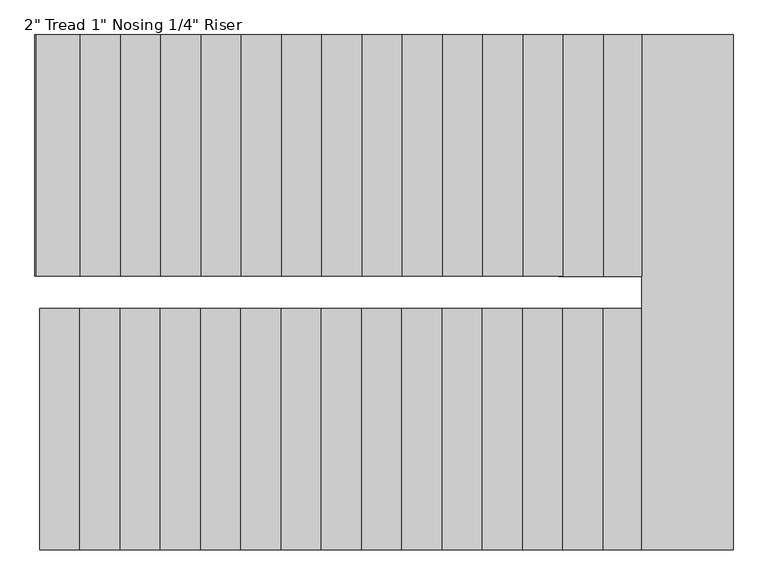
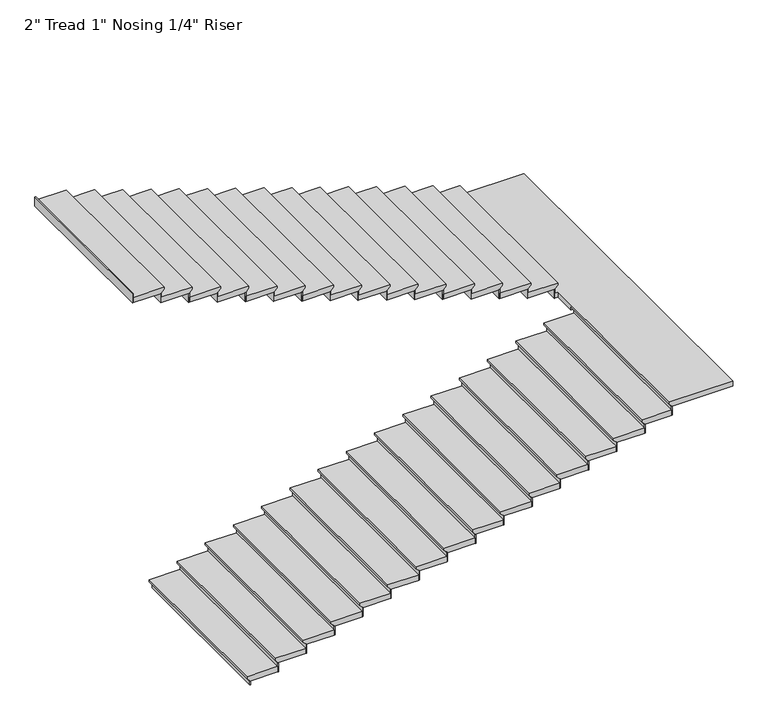
"""IFC4 building model written with IfcOpenShell, lengths in millimetres: stair flight geometry."""

from ifc_helpers import new_model, si_unit, origin, place, context, project, spatial, faceted_brep, source, transform, mapped, element, save


def stair_flight_242bbcd4(model_context):
    return source(origin(), model_context, "Body", "Brep", [
        faceted_brep([(1449.3932247, -2065.2659014, 6162.675), (1449.3932247, -2065.2659014, 6181.725), (1449.3932247, -541.2659014, 6181.725), (1449.3932247, -541.2659014, 6162.675), (1474.7932247, -2065.2659014, 6137.275), (1474.7932247, -541.2659014, 6137.275), (1726.3621616, -2065.2659014, 6181.725), (1726.3621616, -541.2659014, 6181.725), (1474.7932247, -541.2659014, 6130.925), (1726.3621616, -541.2659014, 6130.925), (1726.3621616, -2065.2659014, 6130.925), (1474.7932247, -2065.2659014, 6130.925)], [[[0, 1, 2, 3]], [[4, 0, 3, 5]], [[2, 1, 6, 7]], [[8, 9, 10, 11]], [[2, 7, 9, 8, 5, 3]], [[8, 11, 4, 5]], [[6, 1, 0, 4, 11, 10]], [[7, 6, 10, 9]]]),
        faceted_brep([(1474.7932247, -2065.2659014, 6130.925), (1474.7932247, -2065.2659014, 6096.0), (1481.1432247, -2065.2659014, 6096.0), (1481.1432247, -2065.2659014, 6130.925), (1474.7932247, -541.2659014, 6130.925), (1481.1432247, -541.2659014, 6130.925), (1481.1432247, -541.2659014, 6096.0), (1474.7932247, -541.2659014, 6096.0)], [[[0, 1, 2, 3]], [[4, 5, 6, 7]], [[1, 0, 4, 7]], [[2, 1, 7, 6]], [[3, 2, 6, 5]], [[0, 3, 5, 4]]]),
        faceted_brep([(1726.3621616, -2065.2659014, 6216.65), (1726.3621616, -2065.2659014, 6130.925), (1732.7121616, -2065.2659014, 6130.925), (1732.7121616, -2065.2659014, 6216.65), (1726.3621616, -541.2659014, 6216.65), (1732.7121616, -541.2659014, 6216.65), (1732.7121616, -541.2659014, 6130.925), (1726.3621616, -541.2659014, 6130.925)], [[[0, 1, 2, 3]], [[4, 5, 6, 7]], [[1, 0, 4, 7]], [[2, 1, 7, 6]], [[3, 2, 6, 5]], [[0, 3, 5, 4]]]),
        faceted_brep([(1700.9621616, -541.2659014, 6267.45), (1700.9621616, -2065.2659014, 6267.45), (1980.3621616, -2065.2659014, 6267.45), (1980.3621616, -541.2659014, 6267.45), (1726.3621616, -541.2659014, 6216.65), (1980.3621616, -541.2659014, 6216.65), (1980.3621616, -2065.2659014, 6216.65), (1726.3621616, -2065.2659014, 6216.65), (1726.3621616, -541.2659014, 6223.0), (1700.9621616, -541.2659014, 6248.4), (1726.3621616, -2065.2659014, 6223.0), (1700.9621616, -2065.2659014, 6248.4)], [[[0, 1, 2, 3]], [[4, 5, 6, 7]], [[0, 3, 5, 4, 8, 9]], [[4, 7, 10, 8]], [[2, 1, 11, 10, 7, 6]], [[3, 2, 6, 5]], [[11, 1, 0, 9]], [[10, 11, 9, 8]]]),
        faceted_brep([(1980.3621616, -2065.2659014, 6302.375), (1980.3621616, -2065.2659014, 6216.65), (1986.7121616, -2065.2659014, 6216.65), (1986.7121616, -2065.2659014, 6302.375), (1980.3621616, -541.2659014, 6302.375), (1986.7121616, -541.2659014, 6302.375), (1986.7121616, -541.2659014, 6216.65), (1980.3621616, -541.2659014, 6216.65)], [[[0, 1, 2, 3]], [[4, 5, 6, 7]], [[1, 0, 4, 7]], [[2, 1, 7, 6]], [[3, 2, 6, 5]], [[0, 3, 5, 4]]]),
        faceted_brep([(1954.9621616, -541.2659014, 6353.175), (1954.9621616, -2065.2659014, 6353.175), (2234.3621616, -2065.2659014, 6353.175), (2234.3621616, -541.2659014, 6353.175), (1980.3621616, -541.2659014, 6302.375), (2234.3621616, -541.2659014, 6302.375), (2234.3621616, -2065.2659014, 6302.375), (1980.3621616, -2065.2659014, 6302.375), (1980.3621616, -541.2659014, 6308.725), (1954.9621616, -541.2659014, 6334.125), (1980.3621616, -2065.2659014, 6308.725), (1954.9621616, -2065.2659014, 6334.125)], [[[0, 1, 2, 3]], [[4, 5, 6, 7]], [[0, 3, 5, 4, 8, 9]], [[4, 7, 10, 8]], [[2, 1, 11, 10, 7, 6]], [[3, 2, 6, 5]], [[11, 1, 0, 9]], [[10, 11, 9, 8]]]),
        faceted_brep([(2234.3621616, -2065.2659014, 6388.1), (2234.3621616, -2065.2659014, 6302.375), (2240.7121616, -2065.2659014, 6302.375), (2240.7121616, -2065.2659014, 6388.1), (2234.3621616, -541.2659014, 6388.1), (2240.7121616, -541.2659014, 6388.1), (2240.7121616, -541.2659014, 6302.375), (2234.3621616, -541.2659014, 6302.375)], [[[0, 1, 2, 3]], [[4, 5, 6, 7]], [[1, 0, 4, 7]], [[2, 1, 7, 6]], [[3, 2, 6, 5]], [[0, 3, 5, 4]]]),
        faceted_brep([(2208.9621616, -541.2659014, 6438.9), (2208.9621616, -2065.2659014, 6438.9), (2488.3621616, -2065.2659014, 6438.9), (2488.3621616, -541.2659014, 6438.9), (2234.3621616, -541.2659014, 6388.1), (2488.3621616, -541.2659014, 6388.1), (2488.3621616, -2065.2659014, 6388.1), (2234.3621616, -2065.2659014, 6388.1), (2234.3621616, -541.2659014, 6394.45), (2208.9621616, -541.2659014, 6419.85), (2234.3621616, -2065.2659014, 6394.45), (2208.9621616, -2065.2659014, 6419.85)], [[[0, 1, 2, 3]], [[4, 5, 6, 7]], [[0, 3, 5, 4, 8, 9]], [[4, 7, 10, 8]], [[2, 1, 11, 10, 7, 6]], [[3, 2, 6, 5]], [[11, 1, 0, 9]], [[10, 11, 9, 8]]]),
        faceted_brep([(2488.3621616, -2065.2659014, 6473.825), (2488.3621616, -2065.2659014, 6388.1), (2494.7121616, -2065.2659014, 6388.1), (2494.7121616, -2065.2659014, 6473.825), (2488.3621616, -541.2659014, 6473.825), (2494.7121616, -541.2659014, 6473.825), (2494.7121616, -541.2659014, 6388.1), (2488.3621616, -541.2659014, 6388.1)], [[[0, 1, 2, 3]], [[4, 5, 6, 7]], [[1, 0, 4, 7]], [[2, 1, 7, 6]], [[3, 2, 6, 5]], [[0, 3, 5, 4]]]),
        faceted_brep([(2462.9621616, -541.2659014, 6524.625), (2462.9621616, -2065.2659014, 6524.625), (2742.3621616, -2065.2659014, 6524.625), (2742.3621616, -541.2659014, 6524.625), (2488.3621616, -541.2659014, 6473.825), (2742.3621616, -541.2659014, 6473.825), (2742.3621616, -2065.2659014, 6473.825), (2488.3621616, -2065.2659014, 6473.825), (2488.3621616, -541.2659014, 6480.175), (2462.9621616, -541.2659014, 6505.575), (2488.3621616, -2065.2659014, 6480.175), (2462.9621616, -2065.2659014, 6505.575)], [[[0, 1, 2, 3]], [[4, 5, 6, 7]], [[0, 3, 5, 4, 8, 9]], [[4, 7, 10, 8]], [[2, 1, 11, 10, 7, 6]], [[3, 2, 6, 5]], [[11, 1, 0, 9]], [[10, 11, 9, 8]]]),
        faceted_brep([(2742.3621616, -2065.2659014, 6559.55), (2742.3621616, -2065.2659014, 6473.825), (2748.7121616, -2065.2659014, 6473.825), (2748.7121616, -2065.2659014, 6559.55), (2742.3621616, -541.2659014, 6559.55), (2748.7121616, -541.2659014, 6559.55), (2748.7121616, -541.2659014, 6473.825), (2742.3621616, -541.2659014, 6473.825)], [[[0, 1, 2, 3]], [[4, 5, 6, 7]], [[1, 0, 4, 7]], [[2, 1, 7, 6]], [[3, 2, 6, 5]], [[0, 3, 5, 4]]]),
        faceted_brep([(2716.9621616, -541.2659014, 6610.35), (2716.9621616, -2065.2659014, 6610.35), (2996.3621616, -2065.2659014, 6610.35), (2996.3621616, -541.2659014, 6610.35), (2742.3621616, -541.2659014, 6559.55), (2996.3621616, -541.2659014, 6559.55), (2996.3621616, -2065.2659014, 6559.55), (2742.3621616, -2065.2659014, 6559.55), (2742.3621616, -541.2659014, 6565.9), (2716.9621616, -541.2659014, 6591.3), (2742.3621616, -2065.2659014, 6565.9), (2716.9621616, -2065.2659014, 6591.3)], [[[0, 1, 2, 3]], [[4, 5, 6, 7]], [[0, 3, 5, 4, 8, 9]], [[4, 7, 10, 8]], [[2, 1, 11, 10, 7, 6]], [[3, 2, 6, 5]], [[11, 1, 0, 9]], [[10, 11, 9, 8]]]),
        faceted_brep([(2996.3621616, -2065.2659014, 6645.275), (2996.3621616, -2065.2659014, 6559.55), (3002.7121616, -2065.2659014, 6559.55), (3002.7121616, -2065.2659014, 6645.275), (2996.3621616, -541.2659014, 6645.275), (3002.7121616, -541.2659014, 6645.275), (3002.7121616, -541.2659014, 6559.55), (2996.3621616, -541.2659014, 6559.55)], [[[0, 1, 2, 3]], [[4, 5, 6, 7]], [[1, 0, 4, 7]], [[2, 1, 7, 6]], [[3, 2, 6, 5]], [[0, 3, 5, 4]]]),
        faceted_brep([(2970.9621616, -541.2659014, 6696.075), (2970.9621616, -2065.2659014, 6696.075), (3250.3621616, -2065.2659014, 6696.075), (3250.3621616, -541.2659014, 6696.075), (2996.3621616, -541.2659014, 6645.275), (3250.3621616, -541.2659014, 6645.275), (3250.3621616, -2065.2659014, 6645.275), (2996.3621616, -2065.2659014, 6645.275), (2996.3621616, -541.2659014, 6651.625), (2970.9621616, -541.2659014, 6677.025), (2996.3621616, -2065.2659014, 6651.625), (2970.9621616, -2065.2659014, 6677.025)], [[[0, 1, 2, 3]], [[4, 5, 6, 7]], [[0, 3, 5, 4, 8, 9]], [[4, 7, 10, 8]], [[2, 1, 11, 10, 7, 6]], [[3, 2, 6, 5]], [[11, 1, 0, 9]], [[10, 11, 9, 8]]]),
        faceted_brep([(3250.3621616, -2065.2659014, 6731.0), (3250.3621616, -2065.2659014, 6645.275), (3256.7121616, -2065.2659014, 6645.275), (3256.7121616, -2065.2659014, 6731.0), (3250.3621616, -541.2659014, 6731.0), (3256.7121616, -541.2659014, 6731.0), (3256.7121616, -541.2659014, 6645.275), (3250.3621616, -541.2659014, 6645.275)], [[[0, 1, 2, 3]], [[4, 5, 6, 7]], [[1, 0, 4, 7]], [[2, 1, 7, 6]], [[3, 2, 6, 5]], [[0, 3, 5, 4]]]),
        faceted_brep([(3224.9621616, -541.2659014, 6781.8), (3224.9621616, -2065.2659014, 6781.8), (3504.3621616, -2065.2659014, 6781.8), (3504.3621616, -541.2659014, 6781.8), (3250.3621616, -541.2659014, 6731.0), (3504.3621616, -541.2659014, 6731.0), (3504.3621616, -2065.2659014, 6731.0), (3250.3621616, -2065.2659014, 6731.0), (3250.3621616, -541.2659014, 6737.35), (3224.9621616, -541.2659014, 6762.75), (3250.3621616, -2065.2659014, 6737.35), (3224.9621616, -2065.2659014, 6762.75)], [[[0, 1, 2, 3]], [[4, 5, 6, 7]], [[0, 3, 5, 4, 8, 9]], [[4, 7, 10, 8]], [[2, 1, 11, 10, 7, 6]], [[3, 2, 6, 5]], [[11, 1, 0, 9]], [[10, 11, 9, 8]]]),
        faceted_brep([(3504.3621616, -2065.2659014, 6816.725), (3504.3621616, -2065.2659014, 6731.0), (3510.7121616, -2065.2659014, 6731.0), (3510.7121616, -2065.2659014, 6816.725), (3504.3621616, -541.2659014, 6816.725), (3510.7121616, -541.2659014, 6816.725), (3510.7121616, -541.2659014, 6731.0), (3504.3621616, -541.2659014, 6731.0)], [[[0, 1, 2, 3]], [[4, 5, 6, 7]], [[1, 0, 4, 7]], [[2, 1, 7, 6]], [[3, 2, 6, 5]], [[0, 3, 5, 4]]]),
        faceted_brep([(3478.9621616, -541.2659014, 6867.525), (3478.9621616, -2065.2659014, 6867.525), (3758.3621616, -2065.2659014, 6867.525), (3758.3621616, -541.2659014, 6867.525), (3504.3621616, -541.2659014, 6816.725), (3758.3621616, -541.2659014, 6816.725), (3758.3621616, -2065.2659014, 6816.725), (3504.3621616, -2065.2659014, 6816.725), (3504.3621616, -541.2659014, 6823.075), (3478.9621616, -541.2659014, 6848.475), (3504.3621616, -2065.2659014, 6823.075), (3478.9621616, -2065.2659014, 6848.475)], [[[0, 1, 2, 3]], [[4, 5, 6, 7]], [[0, 3, 5, 4, 8, 9]], [[4, 7, 10, 8]], [[2, 1, 11, 10, 7, 6]], [[3, 2, 6, 5]], [[11, 1, 0, 9]], [[10, 11, 9, 8]]]),
        faceted_brep([(3758.3621616, -2065.2659014, 6902.45), (3758.3621616, -2065.2659014, 6816.725), (3764.7121616, -2065.2659014, 6816.725), (3764.7121616, -2065.2659014, 6902.45), (3758.3621616, -541.2659014, 6902.45), (3764.7121616, -541.2659014, 6902.45), (3764.7121616, -541.2659014, 6816.725), (3758.3621616, -541.2659014, 6816.725)], [[[0, 1, 2, 3]], [[4, 5, 6, 7]], [[1, 0, 4, 7]], [[2, 1, 7, 6]], [[3, 2, 6, 5]], [[0, 3, 5, 4]]]),
        faceted_brep([(3732.9621616, -541.2659014, 6953.25), (3732.9621616, -2065.2659014, 6953.25), (4012.3621616, -2065.2659014, 6953.25), (4012.3621616, -541.2659014, 6953.25), (3758.3621616, -541.2659014, 6902.45), (4012.3621616, -541.2659014, 6902.45), (4012.3621616, -2065.2659014, 6902.45), (3758.3621616, -2065.2659014, 6902.45), (3758.3621616, -541.2659014, 6908.8), (3732.9621616, -541.2659014, 6934.2), (3758.3621616, -2065.2659014, 6908.8), (3732.9621616, -2065.2659014, 6934.2)], [[[0, 1, 2, 3]], [[4, 5, 6, 7]], [[0, 3, 5, 4, 8, 9]], [[4, 7, 10, 8]], [[2, 1, 11, 10, 7, 6]], [[3, 2, 6, 5]], [[11, 1, 0, 9]], [[10, 11, 9, 8]]]),
        faceted_brep([(4012.3621616, -2065.2659014, 6988.175), (4012.3621616, -2065.2659014, 6902.45), (4018.7121616, -2065.2659014, 6902.45), (4018.7121616, -2065.2659014, 6988.175), (4012.3621616, -541.2659014, 6988.175), (4018.7121616, -541.2659014, 6988.175), (4018.7121616, -541.2659014, 6902.45), (4012.3621616, -541.2659014, 6902.45)], [[[0, 1, 2, 3]], [[4, 5, 6, 7]], [[1, 0, 4, 7]], [[2, 1, 7, 6]], [[3, 2, 6, 5]], [[0, 3, 5, 4]]]),
        faceted_brep([(3986.9621616, -541.2659014, 7038.975), (3986.9621616, -2065.2659014, 7038.975), (4266.3621616, -2065.2659014, 7038.975), (4266.3621616, -541.2659014, 7038.975), (4012.3621616, -541.2659014, 6988.175), (4266.3621616, -541.2659014, 6988.175), (4266.3621616, -2065.2659014, 6988.175), (4012.3621616, -2065.2659014, 6988.175), (4012.3621616, -541.2659014, 6994.525), (3986.9621616, -541.2659014, 7019.925), (4012.3621616, -2065.2659014, 6994.525), (3986.9621616, -2065.2659014, 7019.925)], [[[0, 1, 2, 3]], [[4, 5, 6, 7]], [[0, 3, 5, 4, 8, 9]], [[4, 7, 10, 8]], [[2, 1, 11, 10, 7, 6]], [[3, 2, 6, 5]], [[11, 1, 0, 9]], [[10, 11, 9, 8]]]),
        faceted_brep([(4266.3621616, -2065.2659014, 7073.9), (4266.3621616, -2065.2659014, 6988.175), (4272.7121616, -2065.2659014, 6988.175), (4272.7121616, -2065.2659014, 7073.9), (4266.3621616, -541.2659014, 7073.9), (4272.7121616, -541.2659014, 7073.9), (4272.7121616, -541.2659014, 6988.175), (4266.3621616, -541.2659014, 6988.175)], [[[0, 1, 2, 3]], [[4, 5, 6, 7]], [[1, 0, 4, 7]], [[2, 1, 7, 6]], [[3, 2, 6, 5]], [[0, 3, 5, 4]]]),
        faceted_brep([(4240.9621616, -541.2659014, 7124.7), (4240.9621616, -2065.2659014, 7124.7), (4520.3621616, -2065.2659014, 7124.7), (4520.3621616, -541.2659014, 7124.7), (4266.3621616, -541.2659014, 7073.9), (4520.3621616, -541.2659014, 7073.9), (4520.3621616, -2065.2659014, 7073.9), (4266.3621616, -2065.2659014, 7073.9), (4266.3621616, -541.2659014, 7080.25), (4240.9621616, -541.2659014, 7105.65), (4266.3621616, -2065.2659014, 7080.25), (4240.9621616, -2065.2659014, 7105.65)], [[[0, 1, 2, 3]], [[4, 5, 6, 7]], [[0, 3, 5, 4, 8, 9]], [[4, 7, 10, 8]], [[2, 1, 11, 10, 7, 6]], [[3, 2, 6, 5]], [[11, 1, 0, 9]], [[10, 11, 9, 8]]]),
        faceted_brep([(4520.3621616, -2065.2659014, 7159.625), (4520.3621616, -2065.2659014, 7073.9), (4526.7121616, -2065.2659014, 7073.9), (4526.7121616, -2065.2659014, 7159.625), (4520.3621616, -541.2659014, 7159.625), (4526.7121616, -541.2659014, 7159.625), (4526.7121616, -541.2659014, 7073.9), (4520.3621616, -541.2659014, 7073.9)], [[[0, 1, 2, 3]], [[4, 5, 6, 7]], [[1, 0, 4, 7]], [[2, 1, 7, 6]], [[3, 2, 6, 5]], [[0, 3, 5, 4]]]),
        faceted_brep([(4494.9621616, -541.2659014, 7210.425), (4494.9621616, -2065.2659014, 7210.425), (4774.3621616, -2065.2659014, 7210.425), (4774.3621616, -541.2659014, 7210.425), (4520.3621616, -541.2659014, 7159.625), (4774.3621616, -541.2659014, 7159.625), (4774.3621616, -2065.2659014, 7159.625), (4520.3621616, -2065.2659014, 7159.625), (4520.3621616, -541.2659014, 7165.975), (4494.9621616, -541.2659014, 7191.375), (4520.3621616, -2065.2659014, 7165.975), (4494.9621616, -2065.2659014, 7191.375)], [[[0, 1, 2, 3]], [[4, 5, 6, 7]], [[0, 3, 5, 4, 8, 9]], [[4, 7, 10, 8]], [[2, 1, 11, 10, 7, 6]], [[3, 2, 6, 5]], [[11, 1, 0, 9]], [[10, 11, 9, 8]]]),
        faceted_brep([(4774.3621616, -2065.2659014, 7245.35), (4774.3621616, -2065.2659014, 7159.625), (4780.7121616, -2065.2659014, 7159.625), (4780.7121616, -2065.2659014, 7245.35), (4774.3621616, -541.2659014, 7245.35), (4780.7121616, -541.2659014, 7245.35), (4780.7121616, -541.2659014, 7159.625), (4774.3621616, -541.2659014, 7159.625)], [[[0, 1, 2, 3]], [[4, 5, 6, 7]], [[1, 0, 4, 7]], [[2, 1, 7, 6]], [[3, 2, 6, 5]], [[0, 3, 5, 4]]]),
        faceted_brep([(4748.9621616, -541.2659014, 7296.15), (4748.9621616, -2065.2659014, 7296.15), (5028.3621616, -2065.2659014, 7296.15), (5028.3621616, -541.2659014, 7296.15), (4774.3621616, -541.2659014, 7245.35), (5028.3621616, -541.2659014, 7245.35), (5028.3621616, -2065.2659014, 7245.35), (4774.3621616, -2065.2659014, 7245.35), (4774.3621616, -541.2659014, 7251.7), (4748.9621616, -541.2659014, 7277.1), (4774.3621616, -2065.2659014, 7251.7), (4748.9621616, -2065.2659014, 7277.1)], [[[0, 1, 2, 3]], [[4, 5, 6, 7]], [[0, 3, 5, 4, 8, 9]], [[4, 7, 10, 8]], [[2, 1, 11, 10, 7, 6]], [[3, 2, 6, 5]], [[11, 1, 0, 9]], [[10, 11, 9, 8]]]),
        faceted_brep([(5028.3621616, -2065.2659014, 7331.075), (5028.3621616, -2065.2659014, 7245.35), (5034.7121616, -2065.2659014, 7245.35), (5034.7121616, -2065.2659014, 7331.075), (5028.3621616, -541.2659014, 7331.075), (5034.7121616, -541.2659014, 7331.075), (5034.7121616, -541.2659014, 7245.35), (5028.3621616, -541.2659014, 7245.35)], [[[0, 1, 2, 3]], [[4, 5, 6, 7]], [[1, 0, 4, 7]], [[2, 1, 7, 6]], [[3, 2, 6, 5]], [[0, 3, 5, 4]]]),
        faceted_brep([(5002.9621616, -541.2659014, 7381.875), (5002.9621616, -2065.2659014, 7381.875), (5272.0669505, -2065.2659014, 7381.875), (5272.0669505, -541.2659014, 7381.875), (5028.3621616, -541.2659014, 7331.075), (5272.0669505, -541.2659014, 7331.075), (5272.0669505, -2065.2659014, 7331.075), (5028.3621616, -2065.2659014, 7331.075), (5028.3621616, -541.2659014, 7337.425), (5002.9621616, -541.2659014, 7362.825), (5028.3621616, -2065.2659014, 7337.425), (5002.9621616, -2065.2659014, 7362.825)], [[[0, 1, 2, 3]], [[4, 5, 6, 7]], [[0, 3, 5, 4, 8, 9]], [[4, 7, 10, 8]], [[2, 1, 11, 10, 7, 6]], [[3, 2, 6, 5]], [[11, 1, 0, 9]], [[10, 11, 9, 8]]]),
        faceted_brep([(5272.0669505, -2065.2659014, 7416.8), (5272.0669505, -2065.2659014, 7331.075), (5278.4169505, -2065.2659014, 7331.075), (5278.4169505, -2065.2659014, 7416.8), (5272.0669505, -541.2659014, 7416.8), (5278.4169505, -541.2659014, 7416.8), (5278.4169505, -541.2659014, 7331.075), (5272.0669505, -541.2659014, 7331.075)], [[[0, 1, 2, 3]], [[4, 5, 6, 7]], [[1, 0, 4, 7]], [[2, 1, 7, 6]], [[3, 2, 6, 5]], [[0, 3, 5, 4]]]),
        faceted_brep([(5221.2669505, -337.9910016, 7467.6), (5246.6669505, -337.9910016, 7467.6), (5246.6669505, -2065.2659014, 7467.6), (5822.2548051, -2065.2659014, 7467.6), (5822.2548051, 1185.9340986, 7467.6), (5221.2669505, 1185.9340986, 7467.6), (5246.6669505, -337.9910016, 7416.8), (5221.2669505, -337.9910016, 7416.8), (5221.2669505, 1185.9340986, 7416.8), (5822.2548051, 1185.9340986, 7416.8), (5822.2548051, -2065.2659014, 7416.8), (5272.0669505, -2065.2659014, 7416.8), (5272.0669505, -541.2659014, 7416.8), (5246.6669505, -541.2659014, 7416.8), (5246.6669505, -541.2659014, 7448.55), (5246.6669505, -2065.2659014, 7448.55), (5272.0669505, -541.2659014, 7423.15), (5272.0669505, -2065.2659014, 7423.15)], [[[0, 1, 2, 3, 4, 5]], [[6, 7, 8, 9, 10, 11, 12, 13]], [[1, 0, 7, 6]], [[2, 1, 6, 13, 14, 15]], [[13, 12, 16, 14]], [[12, 11, 17, 16]], [[3, 2, 15, 17, 11, 10]], [[4, 3, 10, 9]], [[5, 4, 9, 8]], [[0, 5, 8, 7]], [[17, 15, 14, 16]]]),
        faceted_brep([(5221.2669505, 1185.9340986, 7502.525), (5221.2669505, 1185.9340986, 7416.8), (5214.9169505, 1185.9340986, 7416.8), (5214.9169505, 1185.9340986, 7502.525), (5221.2669505, -337.9910016, 7502.525), (5214.9169505, -337.9910016, 7502.525), (5214.9169505, -337.9910016, 7416.8), (5221.2669505, -337.9910016, 7416.8)], [[[0, 1, 2, 3]], [[4, 5, 6, 7]], [[1, 0, 4, 7]], [[2, 1, 7, 6]], [[3, 2, 6, 5]], [[0, 3, 5, 4]]]),
        faceted_brep([(5246.6669505, -337.9910016, 7553.325), (5246.6669505, 1185.9340986, 7553.325), (4977.5621616, 1185.9340986, 7553.325), (4977.5621616, -337.9910016, 7553.325), (5221.2669505, -337.9910016, 7502.525), (4977.5621616, -337.9910016, 7502.525), (4977.5621616, 1185.9340986, 7502.525), (5221.2669505, 1185.9340986, 7502.525), (5221.2669505, -337.9910016, 7508.875), (5246.6669505, -337.9910016, 7534.275), (5221.2669505, 1185.9340986, 7508.875), (5246.6669505, 1185.9340986, 7534.275)], [[[0, 1, 2, 3]], [[4, 5, 6, 7]], [[0, 3, 5, 4, 8, 9]], [[4, 7, 10, 8]], [[2, 1, 11, 10, 7, 6]], [[3, 2, 6, 5]], [[11, 1, 0, 9]], [[10, 11, 9, 8]]]),
        faceted_brep([(4977.5621616, 1185.9340986, 7588.25), (4977.5621616, 1185.9340986, 7502.525), (4971.2121616, 1185.9340986, 7502.525), (4971.2121616, 1185.9340986, 7588.25), (4977.5621616, -337.9910016, 7588.25), (4971.2121616, -337.9910016, 7588.25), (4971.2121616, -337.9910016, 7502.525), (4977.5621616, -337.9910016, 7502.525)], [[[0, 1, 2, 3]], [[4, 5, 6, 7]], [[1, 0, 4, 7]], [[2, 1, 7, 6]], [[3, 2, 6, 5]], [[0, 3, 5, 4]]]),
        faceted_brep([(5002.9621616, -337.9910016, 7639.05), (5002.9621616, 1185.9340986, 7639.05), (4723.5621616, 1185.9340986, 7639.05), (4723.5621616, -337.9910016, 7639.05), (4977.5621616, -337.9910016, 7588.25), (4723.5621616, -337.9910016, 7588.25), (4723.5621616, 1185.9340986, 7588.25), (4977.5621616, 1185.9340986, 7588.25), (4977.5621616, -337.9910016, 7594.6), (5002.9621616, -337.9910016, 7620.0), (4977.5621616, 1185.9340986, 7594.6), (5002.9621616, 1185.9340986, 7620.0)], [[[0, 1, 2, 3]], [[4, 5, 6, 7]], [[0, 3, 5, 4, 8, 9]], [[4, 7, 10, 8]], [[2, 1, 11, 10, 7, 6]], [[3, 2, 6, 5]], [[11, 1, 0, 9]], [[10, 11, 9, 8]]]),
        faceted_brep([(4723.5621616, 1185.9340986, 7673.975), (4723.5621616, 1185.9340986, 7588.25), (4717.2121616, 1185.9340986, 7588.25), (4717.2121616, 1185.9340986, 7673.975), (4723.5621616, -337.9910016, 7673.975), (4717.2121616, -337.9910016, 7673.975), (4717.2121616, -337.9910016, 7588.25), (4723.5621616, -337.9910016, 7588.25)], [[[0, 1, 2, 3]], [[4, 5, 6, 7]], [[1, 0, 4, 7]], [[2, 1, 7, 6]], [[3, 2, 6, 5]], [[0, 3, 5, 4]]]),
        faceted_brep([(4748.9621616, -337.9910016, 7724.775), (4748.9621616, 1185.9340986, 7724.775), (4469.5621616, 1185.9340986, 7724.775), (4469.5621616, -337.9910016, 7724.775), (4723.5621616, -337.9910016, 7673.975), (4469.5621616, -337.9910016, 7673.975), (4469.5621616, 1185.9340986, 7673.975), (4723.5621616, 1185.9340986, 7673.975), (4723.5621616, -337.9910016, 7680.325), (4748.9621616, -337.9910016, 7705.725), (4723.5621616, 1185.9340986, 7680.325), (4748.9621616, 1185.9340986, 7705.725)], [[[0, 1, 2, 3]], [[4, 5, 6, 7]], [[0, 3, 5, 4, 8, 9]], [[4, 7, 10, 8]], [[2, 1, 11, 10, 7, 6]], [[3, 2, 6, 5]], [[11, 1, 0, 9]], [[10, 11, 9, 8]]]),
        faceted_brep([(4469.5621616, 1185.9340986, 7759.7), (4469.5621616, 1185.9340986, 7673.975), (4463.2121616, 1185.9340986, 7673.975), (4463.2121616, 1185.9340986, 7759.7), (4469.5621616, -337.9910016, 7759.7), (4463.2121616, -337.9910016, 7759.7), (4463.2121616, -337.9910016, 7673.975), (4469.5621616, -337.9910016, 7673.975)], [[[0, 1, 2, 3]], [[4, 5, 6, 7]], [[1, 0, 4, 7]], [[2, 1, 7, 6]], [[3, 2, 6, 5]], [[0, 3, 5, 4]]]),
        faceted_brep([(4494.9621616, -337.9910016, 7810.5), (4494.9621616, 1185.9340986, 7810.5), (4215.5621616, 1185.9340986, 7810.5), (4215.5621616, -337.9910016, 7810.5), (4469.5621616, -337.9910016, 7759.7), (4215.5621616, -337.9910016, 7759.7), (4215.5621616, 1185.9340986, 7759.7), (4469.5621616, 1185.9340986, 7759.7), (4469.5621616, -337.9910016, 7766.05), (4494.9621616, -337.9910016, 7791.45), (4469.5621616, 1185.9340986, 7766.05), (4494.9621616, 1185.9340986, 7791.45)], [[[0, 1, 2, 3]], [[4, 5, 6, 7]], [[0, 3, 5, 4, 8, 9]], [[4, 7, 10, 8]], [[2, 1, 11, 10, 7, 6]], [[3, 2, 6, 5]], [[11, 1, 0, 9]], [[10, 11, 9, 8]]]),
        faceted_brep([(4215.5621616, 1185.9340986, 7845.425), (4215.5621616, 1185.9340986, 7759.7), (4209.2121616, 1185.9340986, 7759.7), (4209.2121616, 1185.9340986, 7845.425), (4215.5621616, -337.9910016, 7845.425), (4209.2121616, -337.9910016, 7845.425), (4209.2121616, -337.9910016, 7759.7), (4215.5621616, -337.9910016, 7759.7)], [[[0, 1, 2, 3]], [[4, 5, 6, 7]], [[1, 0, 4, 7]], [[2, 1, 7, 6]], [[3, 2, 6, 5]], [[0, 3, 5, 4]]]),
        faceted_brep([(4240.9621616, -337.9910016, 7896.225), (4240.9621616, 1185.9340986, 7896.225), (3961.5621616, 1185.9340986, 7896.225), (3961.5621616, -337.9910016, 7896.225), (4215.5621616, -337.9910016, 7845.425), (3961.5621616, -337.9910016, 7845.425), (3961.5621616, 1185.9340986, 7845.425), (4215.5621616, 1185.9340986, 7845.425), (4215.5621616, -337.9910016, 7851.775), (4240.9621616, -337.9910016, 7877.175), (4215.5621616, 1185.9340986, 7851.775), (4240.9621616, 1185.9340986, 7877.175)], [[[0, 1, 2, 3]], [[4, 5, 6, 7]], [[0, 3, 5, 4, 8, 9]], [[4, 7, 10, 8]], [[2, 1, 11, 10, 7, 6]], [[3, 2, 6, 5]], [[11, 1, 0, 9]], [[10, 11, 9, 8]]]),
        faceted_brep([(3961.5621616, 1185.9340986, 7931.15), (3961.5621616, 1185.9340986, 7845.425), (3955.2121616, 1185.9340986, 7845.425), (3955.2121616, 1185.9340986, 7931.15), (3961.5621616, -337.9910016, 7931.15), (3955.2121616, -337.9910016, 7931.15), (3955.2121616, -337.9910016, 7845.425), (3961.5621616, -337.9910016, 7845.425)], [[[0, 1, 2, 3]], [[4, 5, 6, 7]], [[1, 0, 4, 7]], [[2, 1, 7, 6]], [[3, 2, 6, 5]], [[0, 3, 5, 4]]]),
        faceted_brep([(3986.9621616, -337.9910016, 7981.95), (3986.9621616, 1185.9340986, 7981.95), (3707.5621616, 1185.9340986, 7981.95), (3707.5621616, -337.9910016, 7981.95), (3961.5621616, -337.9910016, 7931.15), (3707.5621616, -337.9910016, 7931.15), (3707.5621616, 1185.9340986, 7931.15), (3961.5621616, 1185.9340986, 7931.15), (3961.5621616, -337.9910016, 7937.5), (3986.9621616, -337.9910016, 7962.9), (3961.5621616, 1185.9340986, 7937.5), (3986.9621616, 1185.9340986, 7962.9)], [[[0, 1, 2, 3]], [[4, 5, 6, 7]], [[0, 3, 5, 4, 8, 9]], [[4, 7, 10, 8]], [[2, 1, 11, 10, 7, 6]], [[3, 2, 6, 5]], [[11, 1, 0, 9]], [[10, 11, 9, 8]]]),
        faceted_brep([(3707.5621616, 1185.9340986, 8016.875), (3707.5621616, 1185.9340986, 7931.15), (3701.2121616, 1185.9340986, 7931.15), (3701.2121616, 1185.9340986, 8016.875), (3707.5621616, -337.9910016, 8016.875), (3701.2121616, -337.9910016, 8016.875), (3701.2121616, -337.9910016, 7931.15), (3707.5621616, -337.9910016, 7931.15)], [[[0, 1, 2, 3]], [[4, 5, 6, 7]], [[1, 0, 4, 7]], [[2, 1, 7, 6]], [[3, 2, 6, 5]], [[0, 3, 5, 4]]]),
        faceted_brep([(3732.9621616, -337.9910016, 8067.675), (3732.9621616, 1185.9340986, 8067.675), (3453.5621616, 1185.9340986, 8067.675), (3453.5621616, -337.9910016, 8067.675), (3707.5621616, -337.9910016, 8016.875), (3453.5621616, -337.9910016, 8016.875), (3453.5621616, 1185.9340986, 8016.875), (3707.5621616, 1185.9340986, 8016.875), (3707.5621616, -337.9910016, 8023.225), (3732.9621616, -337.9910016, 8048.625), (3707.5621616, 1185.9340986, 8023.225), (3732.9621616, 1185.9340986, 8048.625)], [[[0, 1, 2, 3]], [[4, 5, 6, 7]], [[0, 3, 5, 4, 8, 9]], [[4, 7, 10, 8]], [[2, 1, 11, 10, 7, 6]], [[3, 2, 6, 5]], [[11, 1, 0, 9]], [[10, 11, 9, 8]]]),
        faceted_brep([(3453.5621616, 1185.9340986, 8102.6), (3453.5621616, 1185.9340986, 8016.875), (3447.2121616, 1185.9340986, 8016.875), (3447.2121616, 1185.9340986, 8102.6), (3453.5621616, -337.9910016, 8102.6), (3447.2121616, -337.9910016, 8102.6), (3447.2121616, -337.9910016, 8016.875), (3453.5621616, -337.9910016, 8016.875)], [[[0, 1, 2, 3]], [[4, 5, 6, 7]], [[1, 0, 4, 7]], [[2, 1, 7, 6]], [[3, 2, 6, 5]], [[0, 3, 5, 4]]]),
        faceted_brep([(3478.9621616, -337.9910016, 8153.4), (3478.9621616, 1185.9340986, 8153.4), (3199.5621616, 1185.9340986, 8153.4), (3199.5621616, -337.9910016, 8153.4), (3453.5621616, -337.9910016, 8102.6), (3199.5621616, -337.9910016, 8102.6), (3199.5621616, 1185.9340986, 8102.6), (3453.5621616, 1185.9340986, 8102.6), (3453.5621616, -337.9910016, 8108.95), (3478.9621616, -337.9910016, 8134.35), (3453.5621616, 1185.9340986, 8108.95), (3478.9621616, 1185.9340986, 8134.35)], [[[0, 1, 2, 3]], [[4, 5, 6, 7]], [[0, 3, 5, 4, 8, 9]], [[4, 7, 10, 8]], [[2, 1, 11, 10, 7, 6]], [[3, 2, 6, 5]], [[11, 1, 0, 9]], [[10, 11, 9, 8]]]),
        faceted_brep([(3199.5621616, 1185.9340986, 8188.325), (3199.5621616, 1185.9340986, 8102.6), (3193.2121616, 1185.9340986, 8102.6), (3193.2121616, 1185.9340986, 8188.325), (3199.5621616, -337.9910016, 8188.325), (3193.2121616, -337.9910016, 8188.325), (3193.2121616, -337.9910016, 8102.6), (3199.5621616, -337.9910016, 8102.6)], [[[0, 1, 2, 3]], [[4, 5, 6, 7]], [[1, 0, 4, 7]], [[2, 1, 7, 6]], [[3, 2, 6, 5]], [[0, 3, 5, 4]]]),
        faceted_brep([(3224.9621616, -337.9910016, 8239.125), (3224.9621616, 1185.9340986, 8239.125), (2945.5621616, 1185.9340986, 8239.125), (2945.5621616, -337.9910016, 8239.125), (3199.5621616, -337.9910016, 8188.325), (2945.5621616, -337.9910016, 8188.325), (2945.5621616, 1185.9340986, 8188.325), (3199.5621616, 1185.9340986, 8188.325), (3199.5621616, -337.9910016, 8194.675), (3224.9621616, -337.9910016, 8220.075), (3199.5621616, 1185.9340986, 8194.675), (3224.9621616, 1185.9340986, 8220.075)], [[[0, 1, 2, 3]], [[4, 5, 6, 7]], [[0, 3, 5, 4, 8, 9]], [[4, 7, 10, 8]], [[2, 1, 11, 10, 7, 6]], [[3, 2, 6, 5]], [[11, 1, 0, 9]], [[10, 11, 9, 8]]]),
        faceted_brep([(2945.5621616, 1185.9340986, 8274.05), (2945.5621616, 1185.9340986, 8188.325), (2939.2121616, 1185.9340986, 8188.325), (2939.2121616, 1185.9340986, 8274.05), (2945.5621616, -337.9910016, 8274.05), (2939.2121616, -337.9910016, 8274.05), (2939.2121616, -337.9910016, 8188.325), (2945.5621616, -337.9910016, 8188.325)], [[[0, 1, 2, 3]], [[4, 5, 6, 7]], [[1, 0, 4, 7]], [[2, 1, 7, 6]], [[3, 2, 6, 5]], [[0, 3, 5, 4]]]),
        faceted_brep([(2970.9621616, -337.9910016, 8324.85), (2970.9621616, 1185.9340986, 8324.85), (2691.5621616, 1185.9340986, 8324.85), (2691.5621616, -337.9910016, 8324.85), (2945.5621616, -337.9910016, 8274.05), (2691.5621616, -337.9910016, 8274.05), (2691.5621616, 1185.9340986, 8274.05), (2945.5621616, 1185.9340986, 8274.05), (2945.5621616, -337.9910016, 8280.4), (2970.9621616, -337.9910016, 8305.8), (2945.5621616, 1185.9340986, 8280.4), (2970.9621616, 1185.9340986, 8305.8)], [[[0, 1, 2, 3]], [[4, 5, 6, 7]], [[0, 3, 5, 4, 8, 9]], [[4, 7, 10, 8]], [[2, 1, 11, 10, 7, 6]], [[3, 2, 6, 5]], [[11, 1, 0, 9]], [[10, 11, 9, 8]]]),
        faceted_brep([(2691.5621616, 1185.9340986, 8359.775), (2691.5621616, 1185.9340986, 8274.05), (2685.2121616, 1185.9340986, 8274.05), (2685.2121616, 1185.9340986, 8359.775), (2691.5621616, -337.9910016, 8359.775), (2685.2121616, -337.9910016, 8359.775), (2685.2121616, -337.9910016, 8274.05), (2691.5621616, -337.9910016, 8274.05)], [[[0, 1, 2, 3]], [[4, 5, 6, 7]], [[1, 0, 4, 7]], [[2, 1, 7, 6]], [[3, 2, 6, 5]], [[0, 3, 5, 4]]]),
        faceted_brep([(2716.9621616, -337.9910016, 8410.575), (2716.9621616, 1185.9340986, 8410.575), (2437.5621616, 1185.9340986, 8410.575), (2437.5621616, -337.9910016, 8410.575), (2691.5621616, -337.9910016, 8359.775), (2437.5621616, -337.9910016, 8359.775), (2437.5621616, 1185.9340986, 8359.775), (2691.5621616, 1185.9340986, 8359.775), (2691.5621616, -337.9910016, 8366.125), (2716.9621616, -337.9910016, 8391.525), (2691.5621616, 1185.9340986, 8366.125), (2716.9621616, 1185.9340986, 8391.525)], [[[0, 1, 2, 3]], [[4, 5, 6, 7]], [[0, 3, 5, 4, 8, 9]], [[4, 7, 10, 8]], [[2, 1, 11, 10, 7, 6]], [[3, 2, 6, 5]], [[11, 1, 0, 9]], [[10, 11, 9, 8]]]),
        faceted_brep([(2437.5621616, 1185.9340986, 8445.5), (2437.5621616, 1185.9340986, 8359.775), (2431.2121616, 1185.9340986, 8359.775), (2431.2121616, 1185.9340986, 8445.5), (2437.5621616, -337.9910016, 8445.5), (2431.2121616, -337.9910016, 8445.5), (2431.2121616, -337.9910016, 8359.775), (2437.5621616, -337.9910016, 8359.775)], [[[0, 1, 2, 3]], [[4, 5, 6, 7]], [[1, 0, 4, 7]], [[2, 1, 7, 6]], [[3, 2, 6, 5]], [[0, 3, 5, 4]]]),
        faceted_brep([(2462.9621616, -337.9910016, 8496.3), (2462.9621616, 1185.9340986, 8496.3), (2183.5621616, 1185.9340986, 8496.3), (2183.5621616, -337.9910016, 8496.3), (2437.5621616, -337.9910016, 8445.5), (2183.5621616, -337.9910016, 8445.5), (2183.5621616, 1185.9340986, 8445.5), (2437.5621616, 1185.9340986, 8445.5), (2437.5621616, -337.9910016, 8451.85), (2462.9621616, -337.9910016, 8477.25), (2437.5621616, 1185.9340986, 8451.85), (2462.9621616, 1185.9340986, 8477.25)], [[[0, 1, 2, 3]], [[4, 5, 6, 7]], [[0, 3, 5, 4, 8, 9]], [[4, 7, 10, 8]], [[2, 1, 11, 10, 7, 6]], [[3, 2, 6, 5]], [[11, 1, 0, 9]], [[10, 11, 9, 8]]]),
        faceted_brep([(2183.5621616, 1185.9340986, 8531.225), (2183.5621616, 1185.9340986, 8445.5), (2177.2121616, 1185.9340986, 8445.5), (2177.2121616, 1185.9340986, 8531.225), (2183.5621616, -337.9910016, 8531.225), (2177.2121616, -337.9910016, 8531.225), (2177.2121616, -337.9910016, 8445.5), (2183.5621616, -337.9910016, 8445.5)], [[[0, 1, 2, 3]], [[4, 5, 6, 7]], [[1, 0, 4, 7]], [[2, 1, 7, 6]], [[3, 2, 6, 5]], [[0, 3, 5, 4]]]),
        faceted_brep([(2208.9621616, -337.9910016, 8582.025), (2208.9621616, 1185.9340986, 8582.025), (1929.5621616, 1185.9340986, 8582.025), (1929.5621616, -337.9910016, 8582.025), (2183.5621616, -337.9910016, 8531.225), (1929.5621616, -337.9910016, 8531.225), (1929.5621616, 1185.9340986, 8531.225), (2183.5621616, 1185.9340986, 8531.225), (2183.5621616, -337.9910016, 8537.575), (2208.9621616, -337.9910016, 8562.975), (2183.5621616, 1185.9340986, 8537.575), (2208.9621616, 1185.9340986, 8562.975)], [[[0, 1, 2, 3]], [[4, 5, 6, 7]], [[0, 3, 5, 4, 8, 9]], [[4, 7, 10, 8]], [[2, 1, 11, 10, 7, 6]], [[3, 2, 6, 5]], [[11, 1, 0, 9]], [[10, 11, 9, 8]]]),
        faceted_brep([(1929.5621616, 1185.9340986, 8616.95), (1929.5621616, 1185.9340986, 8531.225), (1923.2121616, 1185.9340986, 8531.225), (1923.2121616, 1185.9340986, 8616.95), (1929.5621616, -337.9910016, 8616.95), (1923.2121616, -337.9910016, 8616.95), (1923.2121616, -337.9910016, 8531.225), (1929.5621616, -337.9910016, 8531.225)], [[[0, 1, 2, 3]], [[4, 5, 6, 7]], [[1, 0, 4, 7]], [[2, 1, 7, 6]], [[3, 2, 6, 5]], [[0, 3, 5, 4]]]),
        faceted_brep([(1954.9621616, -337.9910016, 8667.75), (1954.9621616, 1185.9340986, 8667.75), (1675.5621616, 1185.9340986, 8667.75), (1675.5621616, -337.9910016, 8667.75), (1929.5621616, -337.9910016, 8616.95), (1675.5621616, -337.9910016, 8616.95), (1675.5621616, 1185.9340986, 8616.95), (1929.5621616, 1185.9340986, 8616.95), (1929.5621616, -337.9910016, 8623.3), (1954.9621616, -337.9910016, 8648.7), (1929.5621616, 1185.9340986, 8623.3), (1954.9621616, 1185.9340986, 8648.7)], [[[0, 1, 2, 3]], [[4, 5, 6, 7]], [[0, 3, 5, 4, 8, 9]], [[4, 7, 10, 8]], [[2, 1, 11, 10, 7, 6]], [[3, 2, 6, 5]], [[11, 1, 0, 9]], [[10, 11, 9, 8]]]),
        faceted_brep([(1675.5621616, 1185.9340986, 8702.675), (1675.5621616, 1185.9340986, 8616.95), (1669.2121616, 1185.9340986, 8616.95), (1669.2121616, 1185.9340986, 8702.675), (1675.5621616, -337.9910016, 8702.675), (1669.2121616, -337.9910016, 8702.675), (1669.2121616, -337.9910016, 8616.95), (1675.5621616, -337.9910016, 8616.95)], [[[0, 1, 2, 3]], [[4, 5, 6, 7]], [[1, 0, 4, 7]], [[2, 1, 7, 6]], [[3, 2, 6, 5]], [[0, 3, 5, 4]]]),
        faceted_brep([(1423.9932247, 1185.9340986, 8788.4), (1423.9932247, 1185.9340986, 8702.675), (1417.6432247, 1185.9340986, 8702.675), (1417.6432247, 1185.9340986, 8788.4), (1423.9932247, -337.9910016, 8788.4), (1417.6432247, -337.9910016, 8788.4), (1417.6432247, -337.9910016, 8702.675), (1423.9932247, -337.9910016, 8702.675)], [[[0, 1, 2, 3]], [[4, 5, 6, 7]], [[1, 0, 4, 7]], [[2, 1, 7, 6]], [[3, 2, 6, 5]], [[0, 3, 5, 4]]]),
        faceted_brep([(1700.9621616, -337.9910016, 8753.475), (1700.9621616, 1185.9340986, 8753.475), (1423.9932247, 1185.9340986, 8753.475), (1423.9932247, -337.9910016, 8753.475), (1675.5621616, -337.9910016, 8702.675), (1423.9932247, -337.9910016, 8702.675), (1423.9932247, 1185.9340986, 8702.675), (1675.5621616, 1185.9340986, 8702.675), (1675.5621616, -337.9910016, 8709.025), (1700.9621616, -337.9910016, 8734.425), (1675.5621616, 1185.9340986, 8709.025), (1700.9621616, 1185.9340986, 8734.425)], [[[0, 1, 2, 3]], [[4, 5, 6, 7]], [[0, 3, 5, 4, 8, 9]], [[4, 7, 10, 8]], [[2, 1, 11, 10, 7, 6]], [[3, 2, 6, 5]], [[11, 1, 0, 9]], [[10, 11, 9, 8]]]),
    ])


if __name__ == "__main__":
    model = new_model("IFC4")
    model_context = context("Model", 3, world=origin())
    ifc_project = project(units=[si_unit("LENGTHUNIT", "METRE", prefix="MILLI")], contexts=[model_context])
    site = spatial("IfcSite", under=ifc_project)
    building = spatial("IfcBuilding", under=site)
    placement = place(None, origin())
    stair_flight_shape = stair_flight_242bbcd4(model_context)
    element("IfcStairFlight", 1, ObjectType="2\" Tread 1\" Nosing 1/4\" Riser", at=placement, inside=building, context=model_context, shape_type="MappedRepresentation", body=[
        mapped(stair_flight_shape, transform((0.0, 0.0, 0.0), x_axis=(1.0, 0.0, 0.0), y_axis=(0.0, 1.0, 0.0), z_axis=(0.0, 0.0, 1.0))),
    ])
    save(model, "model.ifc")
